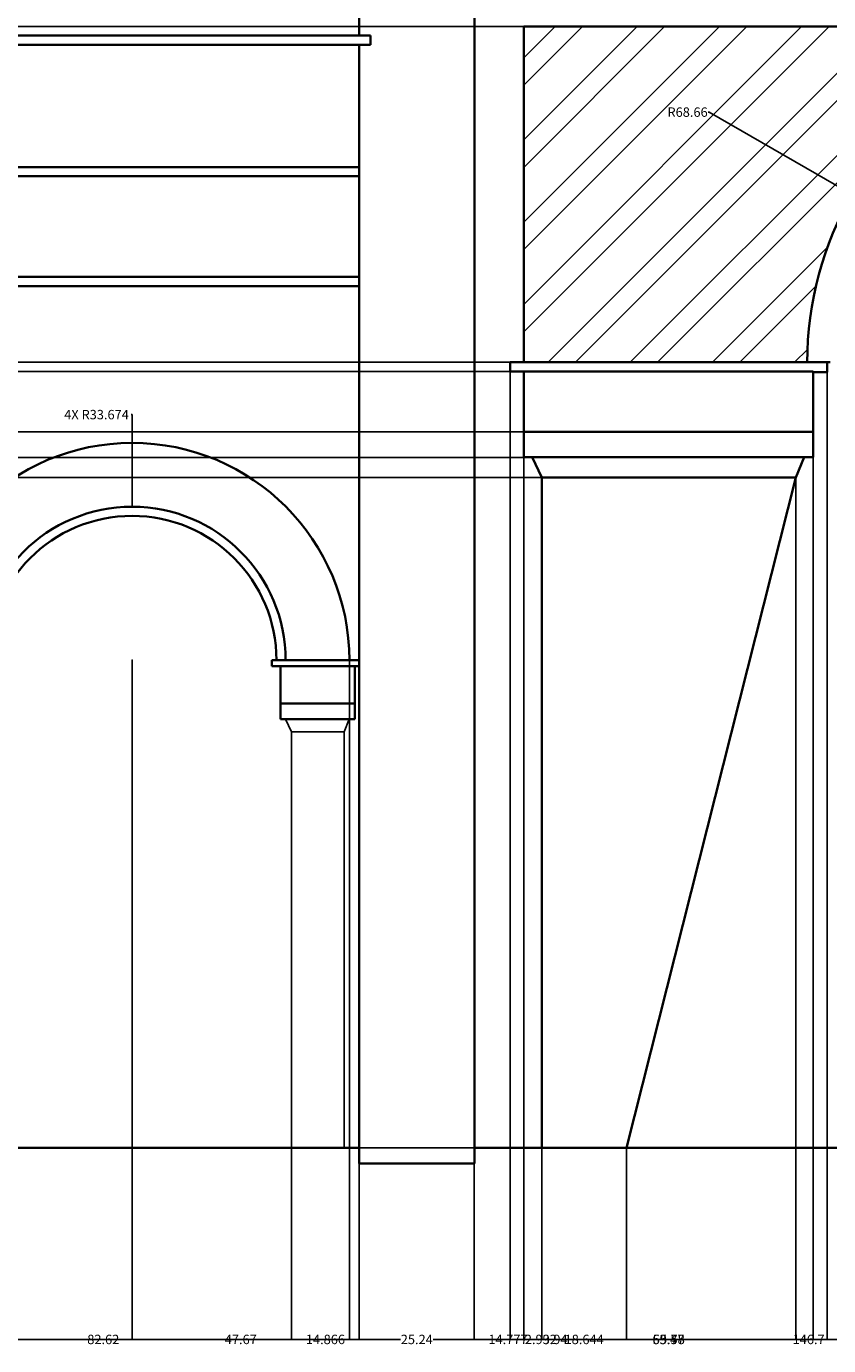
# Model space of a CAD drawing. Units: inches. Extents: x 14 to 859, y 52 to 711.
# Tile 2 of 11: x 190 to 366, y 52 to 342. Entities that reach past the tile are written whole.
import ezdxf

# ---------------------------------------------------------------- set-up
doc = ezdxf.new("R2010")
doc.units = ezdxf.units.IN
doc.header["$MEASUREMENT"] = 0
for name, color, linetype, lineweight in [('A-ANNO-DIMS', 2, 'Continuous', 18), ('A-COLS', 7, 'Continuous', 25), ('A-ELEV', 7, 'Continuous', 35), ('A-ELEV-PATT', 8, 'Continuous', 13)]:
    doc.layers.add(name, color=color, linetype=linetype, lineweight=lineweight)
doc.styles.get("Standard").update_dxf_attribs({"font": 'arial.ttf'})
doc.dimstyles.get("Standard").update_dxf_attribs({"dimtxt": 2.0625, "dimasz": 0.18, "dimexe": 0.18, "dimexo": 0.0625, "dimgap": 0.09, "dimtad": 0, "dimtih": 1, "dimtoh": 1, "dimdec": 4, "dimzin": 0, "dimdsep": 46, "dimlunit": 4, "dimtxsty": 'Standard', "dimcen": 0.09, "dimadec": 0, "dimazin": 0, "dimtfac": 1, "dimtdec": 4, "dimtofl": 0, "dimtmove": 0, "dimatfit": 3, "dimfxl": 1, "dimtolj": 1, "dimtzin": 0, "dimarcsym": 0})

# ---------------------------------------------------------------- blocks, each defined once
blk = doc.blocks.new('COLUMN')
for p, q in [((1.31, 91.21), (0, 93.94)), ((12.88, 91.21), (13.98, 93.94)), ((1.31, 0), (1.31, 91.21)), ((12.88, 91.21), (1.31, 91.21)), ((12.88, 0), (12.88, 91.21))]:
    blk.add_line(p, q)
blk = doc.blocks.new('*D13')
at = {"layer": 'A-ANNO-DIMS', "color": 0, "lineweight": -2, "transparency": 16777216}
for p, q in [((60.78, 339.73), (60.78, 709.71)), ((60.96, 709.53), (432.6, 709.53)), ((811.37, 709.53), (439.73, 709.53)), ((811.55, 339.73), (811.55, 709.71))]:
    blk.add_line(p, q, dxfattribs=at)
at = {"layer": 'A-ANNO-DIMS', "color": 0, "transparency": 16777216}
for points in [[(60.96, 709.56), (60.96, 709.5), (60.78, 709.53)], [(811.37, 709.56), (811.37, 709.5), (811.55, 709.53)]]:
    blk.add_solid(points, dxfattribs=at)
at = {"layer": 'Defpoints', "color": 0, "transparency": 16777216}
for p in [(811.55, 709.53), (60.78, 339.66), (811.55, 339.66)]:
    blk.add_point(p, dxfattribs=at)
at = {"layer": 'A-ANNO-DIMS', "color": 0, "transparency": 16777216, "insert": (436.17, 709.53), "char_height": 2.062, "attachment_point": 5}
blk.add_mtext('\\A1;750.8', dxfattribs=at)
blk = doc.blocks.new('*D14')
at = {"layer": 'A-ANNO-DIMS', "color": 0, "lineweight": -2, "transparency": 16777216}
for p, q in [((262.65, 92.27), (262.65, 53.56)), ((287.89, 92.27), (287.89, 53.56)), ((262.83, 53.74), (271.69, 53.74)), ((287.71, 53.74), (278.86, 53.74))]:
    blk.add_line(p, q, dxfattribs=at)
at = {"layer": 'A-ANNO-DIMS', "color": 0, "transparency": 16777216}
for points in [[(262.83, 53.77), (262.83, 53.71), (262.65, 53.74)], [(287.71, 53.77), (287.71, 53.71), (287.89, 53.74)]]:
    blk.add_solid(points, dxfattribs=at)
at = {"layer": 'Defpoints', "color": 0, "transparency": 16777216}
for p in [(262.65, 92.34), (287.89, 92.34), (287.89, 53.74)]:
    blk.add_point(p, dxfattribs=at)
at = {"layer": 'A-ANNO-DIMS', "color": 0, "transparency": 16777216, "insert": (275.27, 53.74), "char_height": 2.062, "attachment_point": 5}
blk.add_mtext('\\A1;25.24', dxfattribs=at)
blk = doc.blocks.new('*D16')
at = {"layer": 'A-ANNO-DIMS', "color": 0, "lineweight": -2, "transparency": 16777216}
for p, q in [((429.96, 670.76), (17.7, 670.76)), ((17.88, 670.58), (17.88, 384.41)), ((17.88, 95.97), (17.88, 382.14)), ((60.72, 95.79), (17.7, 95.79))]:
    blk.add_line(p, q, dxfattribs=at)
at = {"layer": 'A-ANNO-DIMS', "color": 0, "transparency": 16777216}
for points in [[(17.85, 670.58), (17.91, 670.58), (17.88, 670.76)], [(17.85, 95.97), (17.91, 95.97), (17.88, 95.79)]]:
    blk.add_solid(points, dxfattribs=at)
at = {"layer": 'Defpoints', "color": 0, "transparency": 16777216}
for p in [(17.88, 670.76), (430.02, 670.76), (60.78, 95.79)]:
    blk.add_point(p, dxfattribs=at)
at = {"layer": 'A-ANNO-DIMS', "color": 0, "transparency": 16777216, "insert": (17.88, 383.28), "char_height": 2.062, "attachment_point": 5}
blk.add_mtext('\\A1;575', dxfattribs=at)
blk = doc.blocks.new('*D20')
at = {"layer": 'A-ANNO-DIMS', "color": 0, "lineweight": -2, "transparency": 16777216}
for p, q in [((298.67, 268.01), (17.7, 268.01)), ((17.88, 267.83), (17.88, 183.02)), ((17.88, 95.97), (17.88, 180.77)), ((302.61, 95.79), (17.7, 95.79))]:
    blk.add_line(p, q, dxfattribs=at)
at = {"layer": 'A-ANNO-DIMS', "color": 0, "transparency": 16777216}
for points in [[(17.85, 267.83), (17.91, 267.83), (17.88, 268.01)], [(17.85, 95.97), (17.91, 95.97), (17.88, 95.79)]]:
    blk.add_solid(points, dxfattribs=at)
at = {"layer": 'Defpoints', "color": 0, "transparency": 16777216}
for p in [(17.88, 268.01), (298.73, 268.01), (302.67, 95.79)]:
    blk.add_point(p, dxfattribs=at)
at = {"layer": 'A-ANNO-DIMS', "color": 0, "transparency": 16777216, "insert": (17.88, 181.9), "char_height": 2.062, "attachment_point": 5}
blk.add_mtext('\\A1;172.22', dxfattribs=at)
blk = doc.blocks.new('*D24')
at = {"layer": 'A-ANNO-DIMS', "color": 0, "lineweight": -2, "transparency": 16777216}
for p, q in [((434.6, 267.95), (434.6, 53.56)), ((287.89, 95.73), (287.89, 53.56)), ((288.07, 53.74), (357.77, 53.74)), ((434.42, 53.74), (364.72, 53.74))]:
    blk.add_line(p, q, dxfattribs=at)
at = {"layer": 'A-ANNO-DIMS', "color": 0, "transparency": 16777216}
for points in [[(288.07, 53.77), (288.07, 53.71), (287.89, 53.74)], [(434.42, 53.77), (434.42, 53.71), (434.6, 53.74)]]:
    blk.add_solid(points, dxfattribs=at)
at = {"layer": 'Defpoints', "color": 0, "transparency": 16777216}
for p in [(434.6, 268.01), (287.89, 95.79), (434.6, 53.74)]:
    blk.add_point(p, dxfattribs=at)
at = {"layer": 'A-ANNO-DIMS', "color": 0, "transparency": 16777216, "insert": (361.24, 53.74), "char_height": 2.062, "attachment_point": 5}
blk.add_mtext('\\A1;146.7', dxfattribs=at)
blk = doc.blocks.new('*D25')
at = {"layer": 'A-ANNO-DIMS', "color": 0, "lineweight": -2, "transparency": 16777216}
for p, q in [((298.67, 341.67), (17.7, 341.67)), ((17.88, 341.49), (17.88, 305.98)), ((17.88, 268.19), (17.88, 303.7)), ((298.67, 268.01), (17.7, 268.01))]:
    blk.add_line(p, q, dxfattribs=at)
at = {"layer": 'A-ANNO-DIMS', "color": 0, "transparency": 16777216}
for points in [[(17.85, 341.49), (17.91, 341.49), (17.88, 341.67)], [(17.85, 268.19), (17.91, 268.19), (17.88, 268.01)]]:
    blk.add_solid(points, dxfattribs=at)
at = {"layer": 'Defpoints', "color": 0, "transparency": 16777216}
for p in [(17.88, 341.67), (298.73, 341.67), (298.73, 268.01)]:
    blk.add_point(p, dxfattribs=at)
at = {"layer": 'A-ANNO-DIMS', "color": 0, "transparency": 16777216, "insert": (17.88, 304.84), "char_height": 2.062, "attachment_point": 5}
blk.add_mtext('\\A1;73.66', dxfattribs=at)
blk = doc.blocks.new('*D31')
at = {"layer": 'A-ANNO-DIMS', "color": 0, "lineweight": -2, "transparency": 16777216}
for p, q in [((287.89, 95.73), (287.89, 53.56)), ((302.67, 95.73), (302.67, 53.56)), ((288.07, 53.74), (291.01, 53.74)), ((302.49, 53.74), (299.56, 53.74))]:
    blk.add_line(p, q, dxfattribs=at)
at = {"layer": 'A-ANNO-DIMS', "color": 0, "transparency": 16777216}
for points in [[(288.07, 53.77), (288.07, 53.71), (287.89, 53.74)], [(302.49, 53.77), (302.49, 53.71), (302.67, 53.74)]]:
    blk.add_solid(points, dxfattribs=at)
at = {"layer": 'Defpoints', "color": 0, "transparency": 16777216}
for p in [(287.89, 95.79), (302.67, 95.79), (302.67, 53.74)]:
    blk.add_point(p, dxfattribs=at)
at = {"layer": 'A-ANNO-DIMS', "color": 0, "transparency": 16777216, "insert": (295.28, 53.74), "char_height": 2.062, "attachment_point": 5}
blk.add_mtext('\\A1;14.777', dxfattribs=at)
blk = doc.blocks.new('*D32')
at = {"layer": 'A-ANNO-DIMS', "color": 0, "lineweight": -2, "transparency": 16777216}
for p, q in [((302.67, 95.73), (302.67, 53.56)), ((321.31, 95.73), (321.31, 53.56)), ((302.85, 53.74), (307.72, 53.74)), ((321.13, 53.74), (316.26, 53.74))]:
    blk.add_line(p, q, dxfattribs=at)
at = {"layer": 'A-ANNO-DIMS', "color": 0, "transparency": 16777216}
for points in [[(302.85, 53.77), (302.85, 53.71), (302.67, 53.74)], [(321.13, 53.77), (321.13, 53.71), (321.31, 53.74)]]:
    blk.add_solid(points, dxfattribs=at)
at = {"layer": 'Defpoints', "color": 0, "transparency": 16777216}
for p in [(302.67, 95.79), (321.31, 95.79), (321.31, 53.74)]:
    blk.add_point(p, dxfattribs=at)
at = {"layer": 'A-ANNO-DIMS', "color": 0, "transparency": 16777216, "insert": (311.99, 53.74), "char_height": 2.062, "attachment_point": 5}
blk.add_mtext('\\A1;18.644', dxfattribs=at)
blk = doc.blocks.new('*D35')
at = {"layer": 'A-ANNO-DIMS', "color": 0, "lineweight": -2, "transparency": 16777216}
for p, q in [((298.67, 247.17), (17.7, 247.17)), ((17.88, 246.99), (17.88, 246.12)), ((17.88, 242.95), (17.88, 243.83)), ((302.61, 242.77), (17.7, 242.77))]:
    blk.add_line(p, q, dxfattribs=at)
at = {"layer": 'A-ANNO-DIMS', "color": 0, "transparency": 16777216}
for points in [[(17.85, 246.99), (17.91, 246.99), (17.88, 247.17)], [(17.85, 242.95), (17.91, 242.95), (17.88, 242.77)]]:
    blk.add_solid(points, dxfattribs=at)
at = {"layer": 'Defpoints', "color": 0, "transparency": 16777216}
for p in [(17.88, 247.17), (298.73, 247.17), (302.67, 242.77)]:
    blk.add_point(p, dxfattribs=at)
at = {"layer": 'A-ANNO-DIMS', "color": 0, "transparency": 16777216, "insert": (17.88, 244.97), "char_height": 2.062, "attachment_point": 5}
blk.add_mtext('\\A1;4.397', dxfattribs=at)
blk = doc.blocks.new('*D36')
at = {"layer": 'A-ANNO-DIMS', "color": 0, "lineweight": -2, "transparency": 16777216}
for p, q in [((298.67, 252.78), (17.7, 252.78)), ((17.88, 252.6), (17.88, 251.12)), ((17.88, 247.35), (17.88, 248.83)), ((298.67, 247.17), (17.7, 247.17))]:
    blk.add_line(p, q, dxfattribs=at)
at = {"layer": 'A-ANNO-DIMS', "color": 0, "transparency": 16777216}
for points in [[(17.85, 252.6), (17.91, 252.6), (17.88, 252.78)], [(17.85, 247.35), (17.91, 247.35), (17.88, 247.17)]]:
    blk.add_solid(points, dxfattribs=at)
at = {"layer": 'Defpoints', "color": 0, "transparency": 16777216}
for p in [(17.88, 252.78), (298.73, 252.78), (298.73, 247.17)]:
    blk.add_point(p, dxfattribs=at)
at = {"layer": 'A-ANNO-DIMS', "color": 0, "transparency": 16777216, "insert": (17.88, 249.98), "char_height": 2.062, "attachment_point": 5}
blk.add_mtext('\\A1;5.608', dxfattribs=at)
blk = doc.blocks.new('*D37')
at = {"layer": 'A-ANNO-DIMS', "color": 0, "lineweight": -2, "transparency": 16777216}
for p, q in [((298.67, 265.98), (17.7, 265.98)), ((17.88, 265.8), (17.88, 260.53)), ((17.88, 252.96), (17.88, 258.24)), ((298.67, 252.78), (17.7, 252.78))]:
    blk.add_line(p, q, dxfattribs=at)
at = {"layer": 'A-ANNO-DIMS', "color": 0, "transparency": 16777216}
for points in [[(17.85, 265.8), (17.91, 265.8), (17.88, 265.98)], [(17.85, 252.96), (17.91, 252.96), (17.88, 252.78)]]:
    blk.add_solid(points, dxfattribs=at)
at = {"layer": 'Defpoints', "color": 0, "transparency": 16777216}
for p in [(17.88, 265.98), (298.73, 265.98), (298.73, 252.78)]:
    blk.add_point(p, dxfattribs=at)
at = {"layer": 'A-ANNO-DIMS', "color": 0, "transparency": 16777216, "insert": (17.88, 259.38), "char_height": 2.062, "attachment_point": 5}
blk.add_mtext('\\A1;13.203', dxfattribs=at)
blk = doc.blocks.new('*D38')
at = {"layer": 'A-ANNO-DIMS', "color": 0, "lineweight": -2, "transparency": 16777216}
for p, q in [((295.67, 268.01), (17.7, 268.01)), ((17.88, 268.01), (17.88, 268.19)), ((17.88, 268.19), (18.06, 268.19)), ((17.88, 266.16), (17.88, 267.83)), ((295.67, 265.98), (17.7, 265.98))]:
    blk.add_line(p, q, dxfattribs=at)
at = {"layer": 'A-ANNO-DIMS', "color": 0, "transparency": 16777216}
for points in [[(17.85, 267.83), (17.91, 267.83), (17.88, 268.01)], [(17.85, 266.16), (17.91, 266.16), (17.88, 265.98)]]:
    blk.add_solid(points, dxfattribs=at)
at = {"layer": 'Defpoints', "color": 0, "transparency": 16777216}
for p in [(17.88, 268.01), (295.74, 268.01), (295.74, 265.98)]:
    blk.add_point(p, dxfattribs=at)
at = {"layer": 'A-ANNO-DIMS', "color": 0, "transparency": 16777216, "insert": (21.65, 268.19), "char_height": 2.062, "attachment_point": 5}
blk.add_mtext('\\A1;2.027', dxfattribs=at)
blk = doc.blocks.new('*D39')
at = {"layer": 'A-ANNO-DIMS', "color": 0, "lineweight": -2, "transparency": 16777216}
for p, q in [((298.73, 265.92), (298.73, 53.56)), ((362.2, 265.92), (362.2, 53.56)), ((298.91, 53.74), (326.89, 53.74)), ((362.02, 53.74), (334.04, 53.74))]:
    blk.add_line(p, q, dxfattribs=at)
at = {"layer": 'A-ANNO-DIMS', "color": 0, "transparency": 16777216}
for points in [[(298.91, 53.77), (298.91, 53.71), (298.73, 53.74)], [(362.02, 53.77), (362.02, 53.71), (362.2, 53.74)]]:
    blk.add_solid(points, dxfattribs=at)
at = {"layer": 'Defpoints', "color": 0, "transparency": 16777216}
for p in [(298.73, 265.98), (362.2, 265.98), (362.2, 53.74)]:
    blk.add_point(p, dxfattribs=at)
at = {"layer": 'A-ANNO-DIMS', "color": 0, "transparency": 16777216, "insert": (330.47, 53.74), "char_height": 2.062, "attachment_point": 5}
blk.add_mtext('\\A1;63.47', dxfattribs=at)
blk = doc.blocks.new('*D40')
at = {"layer": 'A-ANNO-DIMS', "color": 0, "lineweight": -2, "transparency": 16777216}
for p, q in [((295.74, 267.95), (295.74, 53.56)), ((365.32, 267.95), (365.32, 53.56)), ((295.92, 53.74), (326.95, 53.74)), ((365.14, 53.74), (334.11, 53.74))]:
    blk.add_line(p, q, dxfattribs=at)
at = {"layer": 'A-ANNO-DIMS', "color": 0, "transparency": 16777216}
for points in [[(295.92, 53.77), (295.92, 53.71), (295.74, 53.74)], [(365.14, 53.77), (365.14, 53.71), (365.32, 53.74)]]:
    blk.add_solid(points, dxfattribs=at)
at = {"layer": 'Defpoints', "color": 0, "transparency": 16777216}
for p in [(295.74, 268.01), (365.32, 268.01), (365.32, 53.74)]:
    blk.add_point(p, dxfattribs=at)
at = {"layer": 'A-ANNO-DIMS', "color": 0, "transparency": 16777216, "insert": (330.53, 53.74), "char_height": 2.062, "attachment_point": 5}
blk.add_mtext('\\A1;69.58', dxfattribs=at)
blk = doc.blocks.new('*D41')
at = {"layer": 'A-ANNO-DIMS', "color": 0, "lineweight": -2, "transparency": 16777216}
for p, q in [((302.67, 242.71), (302.67, 53.56)), ((358.45, 242.71), (358.45, 53.56)), ((302.85, 53.74), (326.99, 53.74)), ((358.27, 53.74), (334.13, 53.74))]:
    blk.add_line(p, q, dxfattribs=at)
at = {"layer": 'A-ANNO-DIMS', "color": 0, "transparency": 16777216}
for points in [[(302.85, 53.77), (302.85, 53.71), (302.67, 53.74)], [(358.27, 53.77), (358.27, 53.71), (358.45, 53.74)]]:
    blk.add_solid(points, dxfattribs=at)
at = {"layer": 'Defpoints', "color": 0, "transparency": 16777216}
for p in [(302.67, 242.77), (358.45, 242.77), (358.45, 53.74)]:
    blk.add_point(p, dxfattribs=at)
at = {"layer": 'A-ANNO-DIMS', "color": 0, "transparency": 16777216, "insert": (330.56, 53.74), "char_height": 2.062, "attachment_point": 5}
blk.add_mtext('\\A1;55.78', dxfattribs=at)
blk = doc.blocks.new('*D42')
at = {"layer": 'A-ANNO-DIMS', "color": 0, "lineweight": -2, "transparency": 16777216}
for p, q in [((295.74, 267.95), (295.74, 53.56)), ((298.73, 265.92), (298.73, 53.56)), ((295.92, 53.74), (298.55, 53.74)), ((298.73, 53.74), (298.91, 53.74))]:
    blk.add_line(p, q, dxfattribs=at)
at = {"layer": 'A-ANNO-DIMS', "color": 0, "transparency": 16777216}
for points in [[(295.92, 53.77), (295.92, 53.71), (295.74, 53.74)], [(298.55, 53.77), (298.55, 53.71), (298.73, 53.74)]]:
    blk.add_solid(points, dxfattribs=at)
at = {"layer": 'Defpoints', "color": 0, "transparency": 16777216}
for p in [(295.74, 268.01), (298.73, 265.98), (298.73, 53.74)]:
    blk.add_point(p, dxfattribs=at)
at = {"layer": 'A-ANNO-DIMS', "color": 0, "transparency": 16777216, "insert": (302.49, 53.74), "char_height": 2.062, "attachment_point": 5}
blk.add_mtext('\\A1;2.992', dxfattribs=at)
blk = doc.blocks.new('*D43')
at = {"layer": 'A-ANNO-DIMS', "color": 0, "lineweight": -2, "transparency": 16777216}
for p, q in [((298.73, 247.11), (298.73, 53.56)), ((302.67, 242.71), (302.67, 53.56)), ((298.91, 53.74), (302.49, 53.74)), ((302.67, 53.74), (302.85, 53.74))]:
    blk.add_line(p, q, dxfattribs=at)
at = {"layer": 'A-ANNO-DIMS', "color": 0, "transparency": 16777216}
for points in [[(298.91, 53.77), (298.91, 53.71), (298.73, 53.74)], [(302.49, 53.77), (302.49, 53.71), (302.67, 53.74)]]:
    blk.add_solid(points, dxfattribs=at)
at = {"layer": 'Defpoints', "color": 0, "transparency": 16777216}
for p in [(298.73, 247.17), (302.67, 242.77), (302.67, 53.74)]:
    blk.add_point(p, dxfattribs=at)
at = {"layer": 'A-ANNO-DIMS', "color": 0, "transparency": 16777216, "insert": (305.61, 53.74), "char_height": 2.062, "attachment_point": 5}
blk.add_mtext('\\A1;3.94', dxfattribs=at)
blk = doc.blocks.new('*D48')
at = {"layer": 'A-ANNO-DIMS', "color": 0, "lineweight": -2, "transparency": 16777216}
for p, q in [((165.17, 95.74), (165.17, 53.56)), ((247.79, 95.73), (247.79, 53.56)), ((165.35, 53.74), (202.92, 53.74)), ((247.61, 53.74), (210.04, 53.74))]:
    blk.add_line(p, q, dxfattribs=at)
at = {"layer": 'A-ANNO-DIMS', "color": 0, "transparency": 16777216}
for points in [[(165.35, 53.77), (165.35, 53.71), (165.17, 53.74)], [(247.61, 53.77), (247.61, 53.71), (247.79, 53.74)]]:
    blk.add_solid(points, dxfattribs=at)
at = {"layer": 'Defpoints', "color": 0, "transparency": 16777216}
for p in [(165.17, 95.8), (247.79, 95.79), (247.79, 53.74)]:
    blk.add_point(p, dxfattribs=at)
at = {"layer": 'A-ANNO-DIMS', "color": 0, "transparency": 16777216, "insert": (206.48, 53.74), "char_height": 2.062, "attachment_point": 5}
blk.add_mtext('\\A1;82.62', dxfattribs=at)
blk = doc.blocks.new('*D49')
at = {"layer": 'A-ANNO-DIMS', "color": 0, "lineweight": -2, "transparency": 16777216}
for p, q in [((247.79, 95.73), (247.79, 53.56)), ((262.65, 95.73), (262.65, 53.56)), ((247.97, 53.74), (250.95, 53.74)), ((262.47, 53.74), (259.49, 53.74))]:
    blk.add_line(p, q, dxfattribs=at)
at = {"layer": 'A-ANNO-DIMS', "color": 0, "transparency": 16777216}
for points in [[(247.97, 53.77), (247.97, 53.71), (247.79, 53.74)], [(262.47, 53.77), (262.47, 53.71), (262.65, 53.74)]]:
    blk.add_solid(points, dxfattribs=at)
at = {"layer": 'Defpoints', "color": 0, "transparency": 16777216}
for p in [(247.79, 95.79), (262.65, 95.79), (262.65, 53.74)]:
    blk.add_point(p, dxfattribs=at)
at = {"layer": 'A-ANNO-DIMS', "color": 0, "transparency": 16777216, "insert": (255.22, 53.74), "char_height": 2.062, "attachment_point": 5}
blk.add_mtext('\\A1;14.866', dxfattribs=at)
blk = doc.blocks.new('*D51')
at = {"layer": 'A-ANNO-DIMS', "color": 0, "lineweight": -2, "transparency": 16777216}
for p, q in [((108.67, 202.6), (108.67, 53.56)), ((212.81, 202.6), (212.81, 53.56)), ((108.85, 53.74), (156.47, 53.74)), ((212.63, 53.74), (165.01, 53.74))]:
    blk.add_line(p, q, dxfattribs=at)
at = {"layer": 'A-ANNO-DIMS', "color": 0, "transparency": 16777216}
for points in [[(108.85, 53.77), (108.85, 53.71), (108.67, 53.74)], [(212.63, 53.77), (212.63, 53.71), (212.81, 53.74)]]:
    blk.add_solid(points, dxfattribs=at)
at = {"layer": 'Defpoints', "color": 0, "transparency": 16777216}
for p in [(108.67, 202.66), (212.81, 202.66), (212.81, 53.74)]:
    blk.add_point(p, dxfattribs=at)
at = {"layer": 'A-ANNO-DIMS', "color": 0, "transparency": 16777216, "insert": (160.74, 53.74), "char_height": 2.062, "attachment_point": 5}
blk.add_mtext('\\A1;104.14', dxfattribs=at)
blk = doc.blocks.new('*D52')
at = {"layer": 'A-ANNO-DIMS', "color": 0, "lineweight": -2, "transparency": 16777216}
for p, q in [((212.81, 202.6), (212.81, 53.56)), ((260.48, 202.6), (260.48, 53.56)), ((212.99, 53.74), (233.04, 53.74)), ((260.3, 53.74), (240.26, 53.74))]:
    blk.add_line(p, q, dxfattribs=at)
at = {"layer": 'A-ANNO-DIMS', "color": 0, "transparency": 16777216}
for points in [[(212.99, 53.77), (212.99, 53.71), (212.81, 53.74)], [(260.3, 53.77), (260.3, 53.71), (260.48, 53.74)]]:
    blk.add_solid(points, dxfattribs=at)
at = {"layer": 'Defpoints', "color": 0, "transparency": 16777216}
for p in [(212.81, 202.66), (260.48, 202.66), (260.48, 53.74)]:
    blk.add_point(p, dxfattribs=at)
at = {"layer": 'A-ANNO-DIMS', "color": 0, "transparency": 16777216, "insert": (236.65, 53.74), "char_height": 2.062, "attachment_point": 5}
blk.add_mtext('\\A1;47.67', dxfattribs=at)
blk = doc.blocks.new('*D126')
at = {"layer": 'A-ANNO-DIMS', "color": 0, "lineweight": -2, "transparency": 16777216}
for p, q in [((339.23, 322.87), (339.41, 322.87)), ((339.41, 322.87), (374.95, 302.39)), ((434.51, 268.01), (434.69, 268.01)), ((434.6, 267.92), (434.6, 268.1))]:
    blk.add_line(p, q, dxfattribs=at)
at = {"layer": 'A-ANNO-DIMS', "color": 0, "transparency": 16777216}
blk.add_solid([(374.97, 302.41), (374.94, 302.36), (375.11, 302.3)], dxfattribs=at)
at = {"layer": 'Defpoints', "color": 0, "transparency": 16777216}
for p in [(375.11, 302.3), (434.6, 268.01)]:
    blk.add_point(p, dxfattribs=at)
at = {"layer": 'A-ANNO-DIMS', "color": 0, "transparency": 16777216, "insert": (334.68, 322.87), "char_height": 2.062, "attachment_point": 5}
blk.add_mtext('\\A1;R68.66', dxfattribs=at)
blk = doc.blocks.new('*D128')
at = {"layer": 'A-ANNO-DIMS', "color": 0, "lineweight": -2, "transparency": 16777216}
for p, q in [((212.61, 256.54), (212.79, 256.54)), ((212.79, 256.54), (212.8, 236.51)), ((212.72, 202.66), (212.9, 202.66)), ((212.81, 202.57), (212.81, 202.75))]:
    blk.add_line(p, q, dxfattribs=at)
at = {"layer": 'A-ANNO-DIMS', "color": 0, "transparency": 16777216}
blk.add_solid([(212.83, 236.51), (212.77, 236.51), (212.8, 236.33)], dxfattribs=at)
at = {"layer": 'Defpoints', "color": 0, "transparency": 16777216}
for p in [(212.8, 236.33), (212.81, 202.66)]:
    blk.add_point(p, dxfattribs=at)
at = {"layer": 'A-ANNO-DIMS', "color": 0, "transparency": 16777216, "insert": (205, 256.54), "char_height": 2.0625, "attachment_point": 5}
blk.add_mtext('\\A1;4X R33.674', dxfattribs=at)

msp = doc.modelspace()

# ---------------------------------------------------------------- hatches: boundary and pattern name
at = {"layer": 'A-ELEV-PATT'}
h = msp.add_hatch(dxfattribs=at)
h.set_pattern_fill('ANSI32', color=256, scale=34)
h.paths.add_polyline_path([(434.5861, 341.6716, 0.41417057), (360.935, 268.0097), (295.7375, 268.0097), (295.7375, 265.9828), (298.7295, 265.9828), (362.2006, 265.9828), (365.3206, 265.8525), (362.2006, 265.8525), (298.7295, 265.9828), (295.7375, 265.9828), (295.7375, 268.0097), (298.7295, 268.0097), (298.7295, 341.6716)])
h.paths.add_polyline_path([(576.5058, 341.6716), (570.5754, 341.6716), (434.5861, 341.6716, -0.41433672), (508.2589, 267.9895), (576.5058, 267.9895)])

# ---------------------------------------------------------------- linework, layer by layer
at = {"layer": 'A-ELEV'}
for p, q in [((287.893, 304.6217), (287.893, 371.6812)), ((262.6537, 339.6626), (262.6537, 370.2389)), ((434.6078, 341.6716), (298.7295, 341.6716)), ((298.7295, 341.6716), (298.7295, 268.0097)), ((60.7804, 339.6626), (262.6537, 339.6626)), ((262.6537, 339.6626), (265.1223, 339.6626)), ((265.1223, 339.6626), (265.1223, 337.6626)), ((60.7804, 337.6626), (262.6537, 337.6626)), ((262.6537, 302.6), (262.6537, 337.6626)), ((265.1223, 337.6626), (262.6537, 337.6626)), ((60.7804, 310.8171), (262.6537, 310.8171)), ((60.7804, 308.8171), (262.6537, 308.8171)), ((287.893, 92.3364), (287.893, 304.6217)), ((262.6537, 202.6598), (262.6537, 302.6)), ((60.7804, 286.7316), (262.6537, 286.7316)), ((60.7804, 284.7316), (262.6537, 284.7316)), ((295.7375, 265.9828), (295.7375, 268.0097)), ((295.7375, 268.0097), (365.935, 268.0097)), ((365.3206, 268.0097), (365.3206, 265.8525)), ((298.7295, 265.9828), (295.7375, 265.9828)), ((298.7295, 252.7801), (298.7295, 265.9828)), ((298.7295, 265.9828), (362.2006, 265.9828)), ((362.2006, 265.9828), (362.2006, 252.7801)), ((365.3206, 265.8525), (362.2006, 265.8525)), ((298.7295, 247.1718), (298.7295, 252.7801)), ((298.7295, 252.7801), (362.2006, 252.7801)), ((362.2006, 252.7801), (362.2006, 247.1718)), ((362.2006, 247.1718), (298.7295, 247.1718)), ((302.6699, 242.7747), (300.5624, 247.1718)), ((358.446, 242.7747), (360.2287, 247.1718)), ((302.6699, 95.7876), (302.6699, 242.7747)), ((358.446, 242.7747), (302.6699, 242.7747)), ((321.3142, 95.7876), (358.446, 242.7747)), ((243.4858, 201.4021), (243.4858, 202.6598)), ((243.4858, 202.6598), (262.6537, 202.6598)), ((262.6537, 202.6598), (262.6537, 92.3364)), ((245.3425, 201.4021), (243.4858, 201.4021)), ((245.3425, 193.2091), (245.3425, 201.4021)), ((245.3425, 201.4021), (261.6873, 201.4021)), ((261.6873, 201.4021), (261.6873, 193.2091)), ((262.6537, 201.4021), (261.6873, 201.4021)), ((245.3425, 189.7289), (245.3425, 193.2091)), ((245.3425, 193.2091), (261.6873, 193.2091)), ((261.6873, 193.2091), (261.6873, 189.7289)), ((261.6873, 189.7289), (245.3425, 189.7289)), ((60.7804, 95.7876), (262.6537, 95.7876)), ((287.893, 95.7876), (584.4409, 95.7876)), ((262.6537, 92.3364), (287.893, 92.3364))]:
    msp.add_line(p, q, dxfattribs=at)
for centre, radius, start in [((434.5969, 268.0097), 73.6619, 359.983178), ((212.8108, 202.6598), 47.6742, 0), ((212.8108, 202.6598), 33.6742, 0), ((212.8108, 202.6598), 31.6742, 0)]:
    msp.add_arc(centre, radius, start, 180, dxfattribs=at)

# ---------------------------------------------------------------- block references
at = {"layer": 'A-COLS'}
msp.add_blockref('COLUMN', (246.4801, 95.788), dxfattribs=at)

# ---------------------------------------------------------------- dimensions: what is measured, and where the dimension line sits
at = {"layer": 'A-ANNO-DIMS'}
for base, p1, p2, override, picture, middle in [((811.5534, 709.5262), (60.7804, 339.6626), (811.5534, 339.6626), {"dimdec": 1, "dimlfac": 1, "dimrnd": 0, "dimzin": 0, "dimdsep": 46, "dimlunit": 2}, '*D13', (436.1669, 709.5262)), ((434.5969, 53.7364), (287.893, 95.7876), (434.5969, 268.0097), {"dimdec": 1, "dimlfac": 1, "dimrnd": 0, "dimzin": 0, "dimdsep": 46, "dimlunit": 2}, '*D24', (361.245, 53.7364)), ((365.3206, 53.7364), (295.7375, 268.0097), (365.3206, 268.0097), {"dimdec": 2, "dimlfac": 1, "dimrnd": 0, "dimzin": 0, "dimdsep": 46, "dimlunit": 2}, '*D40', (330.529, 53.7364)), ((298.7295, 53.7364), (295.7375, 268.0097), (298.7295, 265.9828), {"dimdec": 3, "dimlfac": 1, "dimrnd": 0, "dimzin": 0, "dimdsep": 46, "dimlunit": 2}, '*D42', (302.4865, 53.7364)), ((362.2006, 53.7364), (298.7295, 265.9828), (362.2006, 265.9828), {"dimdec": 2, "dimlfac": 1, "dimrnd": 0, "dimzin": 0, "dimdsep": 46, "dimlunit": 2}, '*D39', (330.4651, 53.7364)), ((302.6699, 53.7364), (298.7295, 247.1718), (302.6699, 242.7747), {"dimdec": 2, "dimlfac": 1, "dimrnd": 0, "dimzin": 0, "dimdsep": 46, "dimlunit": 2}, '*D43', (305.6137, 53.7364)), ((358.446, 53.7364), (302.6699, 242.7747), (358.446, 242.7747), {"dimdec": 2, "dimlfac": 1, "dimrnd": 0, "dimzin": 0, "dimdsep": 46, "dimlunit": 2}, '*D41', (330.5579, 53.7364)), ((212.8108, 53.7364), (108.6715, 202.6598), (212.8108, 202.6598), {"dimdec": 2, "dimlfac": 1, "dimrnd": 0, "dimzin": 0, "dimdsep": 46, "dimlunit": 2}, '*D51', (160.7412, 53.7364)), ((260.4849, 53.7364), (212.8108, 202.6598), (260.4849, 202.6598), {"dimdec": 2, "dimlfac": 1, "dimrnd": 0, "dimzin": 0, "dimdsep": 46, "dimlunit": 2}, '*D52', (236.6479, 53.7364)), ((247.7877, 53.7364), (165.1652, 95.8039), (247.7877, 95.7876), {"dimdec": 2, "dimlfac": 1, "dimrnd": 0, "dimzin": 0, "dimdsep": 46, "dimlunit": 2}, '*D48', (206.4765, 53.7364)), ((262.6537, 53.7364), (247.7877, 95.7876), (262.6537, 95.7876), {"dimdec": 3, "dimlfac": 1, "dimrnd": 0, "dimzin": 0, "dimdsep": 46, "dimlunit": 2}, '*D49', (255.2207, 53.7364)), ((302.6699, 53.7364), (287.893, 95.7876), (302.6699, 95.7876), {"dimdec": 3, "dimlfac": 1, "dimrnd": 0, "dimzin": 0, "dimdsep": 46, "dimlunit": 2}, '*D31', (295.2814, 53.7364)), ((321.3142, 53.7364), (302.6699, 95.7876), (321.3142, 95.7876), {"dimdec": 3, "dimlfac": 1, "dimrnd": 0, "dimzin": 0, "dimdsep": 46, "dimlunit": 2}, '*D32', (311.992, 53.7364)), ((287.893, 53.7364), (262.6537, 92.3364), (287.893, 92.3364), {"dimdec": 2, "dimlfac": 1, "dimrnd": 0, "dimzin": 0, "dimdsep": 46, "dimlunit": 2}, '*D14', (275.2733, 53.7364))]:
    dim = msp.add_linear_dim(base=base, p1=p1, p2=p2, dimstyle='Standard', override=override, dxfattribs=at)
    dim.commit()
    dim.dimension.update_dxf_attribs({"geometry": picture, "text_midpoint": middle})
for base, p1, p2, override, picture, middle in [((17.8785, 670.7637), (60.7804, 95.7876), (430.0228, 670.7637), {"dimdec": 0, "dimlfac": 1, "dimrnd": 0, "dimzin": 0, "dimdsep": 46, "dimlunit": 2}, '*D16', (17.8785, 383.2756)), ((17.8785, 341.6716), (298.7295, 268.0097), (298.7295, 341.6716), {"dimdec": 2, "dimlfac": 1, "dimrnd": 0, "dimzin": 0, "dimdsep": 46, "dimlunit": 2}, '*D25', (17.8785, 304.8406)), ((17.8785, 268.0097), (295.7375, 265.9828), (295.7375, 268.0097), {"dimdec": 3, "dimlfac": 1, "dimrnd": 0, "dimzin": 0, "dimdsep": 46, "dimlunit": 2}, '*D38', (21.646, 268.1897)), ((17.8785, 268.0097), (302.6699, 95.7876), (298.7295, 268.0097), {"dimdec": 2, "dimlfac": 1, "dimrnd": 0, "dimzin": 0, "dimdsep": 46, "dimlunit": 2}, '*D20', (17.8785, 181.8987)), ((17.8785, 265.9828), (298.7295, 252.7801), (298.7295, 265.9828), {"dimdec": 3, "dimlfac": 1, "dimrnd": 0, "dimzin": 0, "dimdsep": 46, "dimlunit": 2}, '*D37', (17.8785, 259.3815)), ((17.8785, 252.7801), (298.7295, 247.1718), (298.7295, 252.7801), {"dimdec": 3, "dimlfac": 1, "dimrnd": 0, "dimzin": 0, "dimdsep": 46, "dimlunit": 2}, '*D36', (17.8785, 249.9759)), ((17.8785, 247.1718), (302.6699, 242.7747), (298.7295, 247.1718), {"dimdec": 3, "dimlfac": 1, "dimrnd": 0, "dimzin": 0, "dimdsep": 46, "dimlunit": 2}, '*D35', (17.8785, 244.9732))]:
    dim = msp.add_linear_dim(base=base, p1=p1, p2=p2, angle=90, dimstyle='Standard', override=override, dxfattribs=at)
    dim.commit()
    dim.dimension.update_dxf_attribs({"geometry": picture, "text_midpoint": middle})
dim = msp.add_radius_dim(center=(434.5969, 268.0097), mpoint=(375.1079, 302.2955), dimstyle='Standard', override={"dimdec": 2, "dimlfac": 1, "dimrnd": 0, "dimzin": 0, "dimdsep": 46, "dimlunit": 2}, dxfattribs=at)
dim.commit()
dim.dimension.update_dxf_attribs({"geometry": '*D126', "text_midpoint": (334.6783, 322.8669), "dimtype": 164})
dim = msp.add_radius_dim(center=(212.8108, 202.6598), mpoint=(212.8, 236.334), text='4X <>', dimstyle='Standard', override={"dimdec": 3, "dimlfac": 1, "dimrnd": 0, "dimzin": 0, "dimdsep": 46, "dimlunit": 2}, dxfattribs=at)
dim.commit()
dim.dimension.update_dxf_attribs({"geometry": '*D128', "text_midpoint": (205.0023, 256.5385), "dimtype": 164})

doc.saveas('drawing.dxf')
